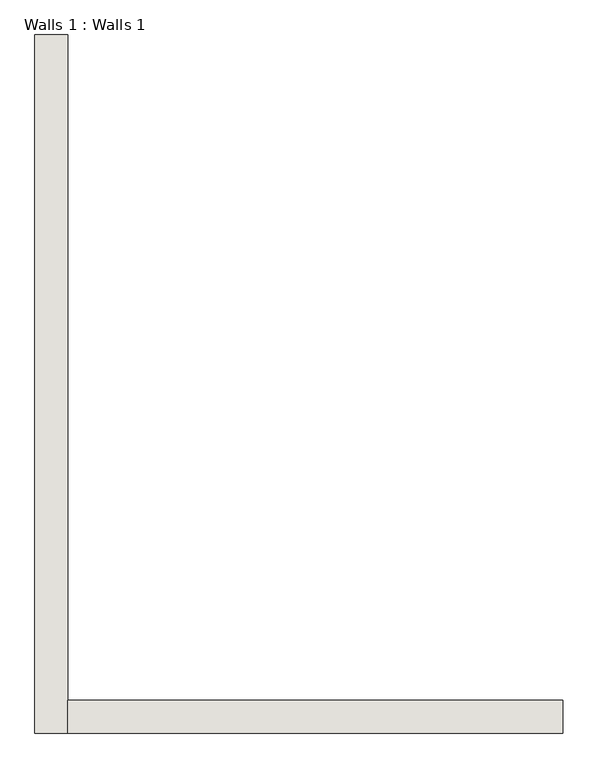
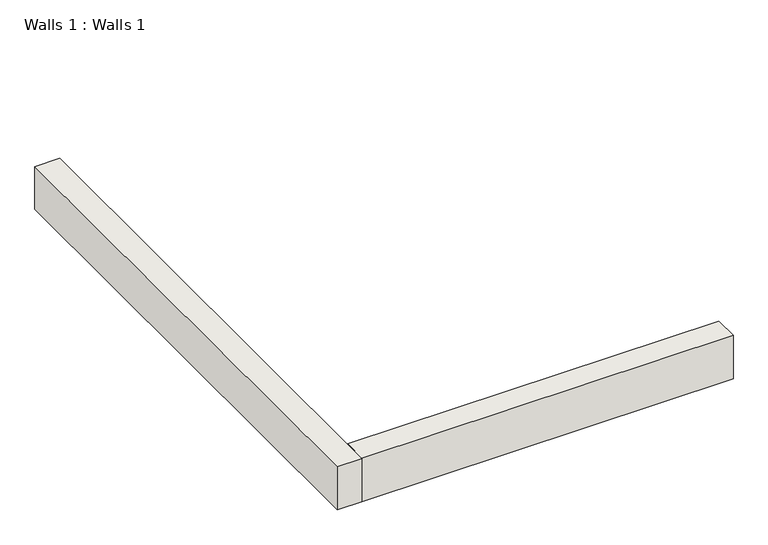
"""IFC4 building model written with IfcOpenShell, lengths in millimetres: wall geometry, Walls 1 : Walls 1."""

from ifc_helpers import new_model, si_unit, frame, origin, place, context, project, spatial, polyline, outline, extrude, source, transform, mapped, element, save


def walls_1_walls_1_c089fa37(model_context):
    return source(origin(), model_context, "Body", "SweptSolid", [
        extrude(outline(polyline([(-12649.8932708, 334.4609482), (-12649.8932708, 6786.0609482), (-12345.0932708, 6786.0609482), (-12345.0932708, 334.4609482), (-12649.8932708, 334.4609482)])), frame((0.0, 0.0, 3657.6), z_axis=(0.0, 0.0, 1.0), x_axis=(1.0, 0.0, 0.0)), (0.0, 0.0, 1.0), 556.583005),
        extrude(outline(polyline([(-7773.0932708, 334.4609482), (-12345.0932708, 334.4609482), (-12345.0932708, 639.2609482), (-7773.0932708, 639.2609482), (-7773.0932708, 334.4609482)])), frame((0.0, 0.0, 3657.6), z_axis=(0.0, 0.0, 1.0), x_axis=(1.0, 0.0, 0.0)), (0.0, 0.0, 1.0), 564.6567089),
    ])


if __name__ == "__main__":
    model = new_model("IFC4")
    model_context = context("Model", 3, world=origin())
    ifc_project = project(units=[si_unit("LENGTHUNIT", "METRE", prefix="MILLI")], contexts=[model_context])
    site = spatial("IfcSite", under=ifc_project)
    building = spatial("IfcBuilding", under=site)
    placement = place(None, origin())
    walls_1_walls_1_shape = walls_1_walls_1_c089fa37(model_context)
    element("IfcWall", 1, ObjectType="Walls 1 : Walls 1", at=placement, inside=building, context=model_context, shape_type="MappedRepresentation", body=[
        mapped(walls_1_walls_1_shape, transform((0.0, 0.0, 0.0), x_axis=(1.0, 0.0, 0.0), y_axis=(0.0, 1.0, 0.0), z_axis=(0.0, 0.0, 1.0))),
    ])
    save(model, "model.ifc")

# Revit data of these elements
# Element 1 (IfcWall, "Walls 1 : Walls 1")
#   Materials on its faces: "Default Wall"
# Materials
#   "Default Wall": colour RGB 128 128 128, transparency 0
